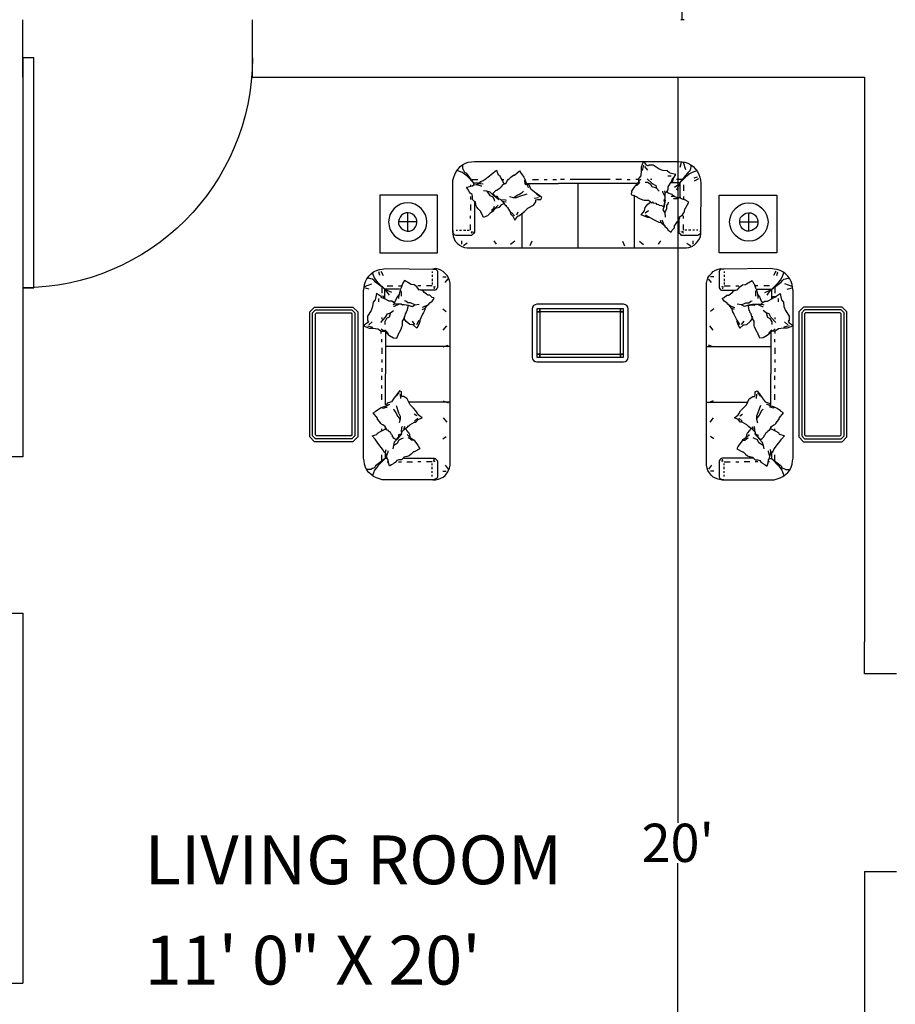
# Model space of a CAD drawing. Units: inches. Extents: x -113 to 5399, y -1393 to 3302.
# Tile 25 of 40: x 3844 to 3982, y 34 to 189. Entities that reach past the tile are written whole.
import ezdxf

# ---------------------------------------------------------------- set-up
doc = ezdxf.new("R2010")
doc.units = ezdxf.units.IN
doc.header["$MEASUREMENT"] = 0
doc.layers.add('24', color=7, linetype='Continuous')
for name, color, linetype, lineweight in [('A-ANNO-DIMS', 254, 'Continuous', 18), ('A-AREA-IDEN', 4, 'Continuous', 18), ('doors', 2, 'Continuous', 25), ('furniture', 131, 'Continuous', 18), ('walls', 1, 'Continuous', 25)]:
    doc.layers.add(name, color=color, linetype=linetype, lineweight=lineweight)
doc.styles.get("Standard").update_dxf_attribs({"font": 'arial.ttf'})
doc.dimstyles.get("Standard").update_dxf_attribs({"dimtxt": 6, "dimasz": 0.18, "dimexe": 0.18, "dimexo": 0.0625, "dimgap": 0.09, "dimtad": 0, "dimtih": 1, "dimtoh": 1, "dimdec": 1, "dimzin": 0, "dimdsep": 46, "dimlunit": 4, "dimtxsty": 'Standard', "dimblk": 'ARCHTICK', "dimcen": 0.09, "dimadec": 0, "dimazin": 0, "dimtfac": 1, "dimtdec": 1, "dimtofl": 0, "dimtmove": 0, "dimatfit": 3, "dimfxl": 1, "dimtolj": 1, "dimtzin": 0, "dimarcsym": 0})

# ---------------------------------------------------------------- blocks, each defined once
blk = doc.blocks.new('*U3')
for p, q in [((0, 0), (0, -6)), ((36, 0), (36, -6))]:
    blk.add_line(p, q)
blk.add_lwpolyline([(0, 0), (0, 36), (1.75, 36), (1.75, 0)], close=True)
blk.add_arc((0, 0), 36, 0, 90)
blk = doc.blocks.new('DL13712')
at = {"layer": '24'}
for p, q in [((33, 28.5), (-34, 28.5)), ((33.5, -29.5), (-10, -29.5))]:
    blk.add_line(p, q, dxfattribs=at)
blk = doc.blocks.new('DL13976')
at = {"layer": '24'}
for p, q in [((-18, 7.5), (-16, 11)), ((-16, 11), (-13.5, 14)), ((-13.5, 14), (-10.5, 16.5)), ((-10.5, 16.5), (-7, 18.5)), ((-7, 18.5), (-3.5, 19.5)), ((-3.5, 19.5), (0.5, 20)), ((0.5, 20), (4.5, 19.5)), ((4.5, 19.5), (8, 18.5)), ((8, 18.5), (11.5, 16.5)), ((11.5, 16.5), (14.5, 14)), ((14.5, 14), (17, 11)), ((17, 11), (19, 7.5)), ((-19.5, 0), (-19, 4)), ((-19, -4), (-19.5, 0)), ((-19, 4), (-18, 7.5)), ((-9, 2), (-8, 4.5)), ((-9, -0.5), (-9, 2)), ((-9, 0), (10, 0)), ((-8, 4.5), (-6.5, 6.5)), ((-6.5, 6.5), (-4.5, 8)), ((-5.5, 0), (6.5, 0)), ((-4.5, 8), (-2.5, 9)), ((-2.5, 9), (0, 9.5)), ((0, 9.5), (2.5, 9.5)), ((0.5, -9.5), (0.5, 9.5)), ((0.5, -6), (0.5, 6)), ((2.5, 9.5), (5, 8.5)), ((5, 8.5), (7, 7)), ((7, 7), (8.5, 5)), ((8.5, 5), (9.5, 3)), ((9.5, 3), (10, 0.5)), ((10, 0.5), (10, -2)), ((19, 7.5), (20, 4)), ((20, 4), (20.5, 0)), ((20.5, 0), (20, -4)), ((-18, -7.5), (-19, -4)), ((-16, -11), (-18, -7.5)), ((-8.5, -3), (-9, -0.5)), ((-7.5, -5), (-8.5, -3)), ((-6, -7), (-7.5, -5)), ((-4, -8.5), (-6, -7)), ((-1.5, -9.5), (-4, -8.5)), ((1, -9.5), (-1.5, -9.5)), ((3.5, -9), (1, -9.5)), ((5.5, -8), (3.5, -9)), ((7.5, -6.5), (5.5, -8)), ((9, -4.5), (7.5, -6.5)), ((10, -2), (9, -4.5)), ((19, -7.5), (17, -11)), ((20, -4), (19, -7.5)), ((-13.5, -14), (-16, -11)), ((-10.5, -16.5), (-13.5, -14)), ((-7, -18.5), (-10.5, -16.5)), ((-3.5, -19.5), (-7, -18.5)), ((0.5, -20), (-3.5, -19.5)), ((4.5, -19.5), (0.5, -20)), ((8, -18.5), (4.5, -19.5)), ((11.5, -16.5), (8, -18.5)), ((14.5, -14), (11.5, -16.5)), ((17, -11), (14.5, -14))]:
    blk.add_line(p, q, dxfattribs=at)
blk = doc.blocks.new('DL13329')
at = {"layer": '24'}
for p, q in [((0, 0), (0, -60)), ((60, 0), (0, 0)), ((60, -60), (60, 0)), ((0, -60), (60, -60))]:
    blk.add_line(p, q, dxfattribs=at)
blk = doc.blocks.new('DL13303')
at = {"layer": '24'}
for p, q in [((-70, 20), (-65, 25)), ((-67, 19), (-64, 22)), ((-65, 25), (65, 25)), ((-64, 22), (64, 22)), ((64, 22), (67, 19)), ((65, 25), (70, 20)), ((-70, -20), (-70, 20)), ((-67, -19), (-67, 19)), ((-64, 18), (-63, 19)), ((-64, -18), (-64, 18)), ((-63, 19), (63, 19)), ((63, 19), (64, 18)), ((64, 18), (64, -18)), ((67, 19), (67, -19)), ((70, 20), (70, -20)), ((-65, -25), (-70, -20)), ((-64, -22), (-67, -19)), ((-63, -19), (-64, -18)), ((63, -19), (-63, -19)), ((64, -18), (63, -19)), ((67, -19), (64, -22)), ((70, -20), (65, -25)), ((65, -25), (-65, -25)), ((64, -22), (-64, -22))]:
    blk.add_line(p, q, dxfattribs=at)
blk = doc.blocks.new('DL12701')
at = {"layer": '24'}
for p, q in [((-102, 40), (-99.5, 42)), ((-99.5, 42), (-96.5, 43.5)), ((-99, 40), (-99, 42)), ((-96.5, 43.5), (-93.5, 44.5)), ((-93.5, 44.5), (-90, 45)), ((-90, 45), (-87, 45.5)), ((-87, 45.5), (0, 45.5)), ((0, 45.5), (87, 45.5)), ((50, 45), (48, 39.5)), ((50.5, 41.5), (49, 36)), ((51.5, 44.5), (50, 45)), ((53.5, 41.5), (51.5, 44.5)), ((55.5, 40.5), (53.5, 41.5)), ((56, 41.5), (55.5, 40.5)), ((60.5, 41.5), (56, 41.5)), ((66.5, 37.5), (60.5, 41.5)), ((87, 45.5), (90.5, 45)), ((88.5, 39.5), (90, 44.5)), ((90.5, 45), (93.5, 44.5)), ((91.5, 44.5), (94, 37)), ((93.5, 44.5), (96.5, 43.5)), ((96.5, 43.5), (99.5, 42)), ((99.5, 42), (102, 40)), ((100, 40), (99.5, 42)), ((-108.5, 29), (-107.5, 32)), ((-107.5, 32), (-106, 35)), ((-106, 35), (-104, 37.5)), ((-102.5, 35), (-105, 36)), ((-104, 37.5), (-102, 40)), ((-99.5, 34), (-102.5, 35)), ((-97, 32), (-99.5, 34)), ((-99, 38), (-99, 40)), ((-98, 36), (-99, 38)), ((-97, 34), (-98, 36)), ((-95, 33), (-97, 34)), ((-95, 30.5), (-97, 32)), ((-87.5, 23), (-95, 33)), ((-71.5, 30.5), (-69.5, 32)), ((-69.5, 32), (-67.5, 33.5)), ((-67.5, 33.5), (-64, 36.5)), ((-64, 36.5), (-62.5, 31.5)), ((-62.5, 31.5), (-61, 31)), ((-61, 31), (-59.5, 28)), ((-49, 29), (-46.5, 31)), ((-46.5, 31), (-45.5, 31)), ((-45.5, 31), (-40, 35.5)), ((-40, 35.5), (-38.5, 33)), ((-38.5, 33), (-38, 32.5)), ((-38, 32.5), (-35.5, 29)), ((48, 35.5), (47.5, 30.5)), ((48, 39.5), (48, 35.5)), ((51.5, 40), (54.5, 36.5)), ((70.5, 36), (66.5, 37.5)), ((75, 35.5), (70.5, 36)), ((77.5, 33.5), (75, 35.5)), ((79, 33), (77.5, 33.5)), ((84, 32), (79, 33)), ((81.5, 28), (84, 32)), ((88.5, 23.5), (96, 33)), ((95.5, 30.5), (98, 32.5)), ((96, 33), (97.5, 34.5)), ((97.5, 34.5), (99, 36)), ((98, 32.5), (100.5, 34)), ((99, 36), (99.5, 38)), ((99.5, 38), (100, 40)), ((100.5, 34), (103, 35)), ((102, 40), (104.5, 37.5)), ((103, 35), (106, 36)), ((104.5, 37.5), (106.5, 35)), ((106.5, 35), (108, 32)), ((108, 32), (109, 29)), ((-109.5, 26), (-108.5, 29)), ((-109.5, 22.5), (-109.5, 26)), ((-109.5, -26.5), (-109.5, 22.5)), ((-87.5, 23), (-95, 30.5)), ((-91, 21), (-91, 19.5)), ((-89.5, 26.5), (-83.5, 26.5)), ((-89, 20), (-87.5, 21)), ((-87.5, 21), (-87.5, 23)), ((-81.5, 23), (-87.5, 23)), ((-87.5, 21), (-85, 21.5)), ((-85, 21.5), (-82, 22.5)), ((-85, 21.5), (-80.5, 20)), ((-82, 22.5), (-80.5, 24.5)), ((-82, 22.5), (-80.5, 22.5)), ((-80.5, 24.5), (-78, 25.5)), ((-80.5, 24.5), (-80.5, 23.5)), ((-80.5, 22.5), (-78, 22)), ((-78, 25.5), (-76, 27)), ((-77, 25.5), (-77, 25.5)), ((-76, 27), (-71.5, 30.5)), ((-59.5, 28), (-57.5, 24.5)), ((-58.5, 19.5), (-58, 21)), ((-58, 26.5), (-56.5, 26.5)), ((-58, 21), (-54.5, 23)), ((-57.5, 24.5), (-56.5, 22)), ((-56.5, 22.5), (-54.5, 22.5)), ((-54.5, 22.5), (-52.5, 25.5)), ((-54.5, 23), (-54.5, 22.5)), ((-54, 22.5), (-54, 22.5)), ((-52.5, 25.5), (-52, 26.5)), ((-52, 26.5), (-51, 27.5)), ((-51, 27.5), (-49, 29)), ((-35.5, 29), (-34.5, 27)), ((-34.5, 27), (-35, 24.5)), ((-35, 24.5), (-34.5, 23)), ((-34.5, 27), (-33.5, 24)), ((-34.5, 23), (-34, 21)), ((-33.5, 24), (-33, 22)), ((-30, 21), (-33, 22)), ((-33, 22), (-31.5, 19.5)), ((-32, 22.5), (0.5, 22.5)), ((-29.5, 19.5), (-30, 21)), ((-26.5, 26.5), (-20.5, 26.5)), ((-14.5, 26.5), (-11.5, 26.5)), ((-5.5, 26.5), (-1.5, 26.5)), ((44, 22.5), (0.5, 22.5)), ((6.5, 26.5), (2.5, 26.5)), ((15.5, 26.5), (12.5, 26.5)), ((27.5, 26.5), (21.5, 26.5)), ((33.5, 26.5), (36.5, 26.5)), ((43.5, 22), (41.5, 20)), ((43.5, 20.5), (41.5, 20)), ((42.5, 27), (45, 27)), ((45, 23.5), (43.5, 22)), ((45, 22), (43.5, 20.5)), ((45.5, 28), (45, 27)), ((45, 27), (45, 23.5)), ((45, 23.5), (46.5, 26)), ((46.5, 23.5), (45, 22)), ((47.5, 30.5), (45.5, 28)), ((46.5, 26), (47.5, 27)), ((54.5, 23.5), (52, 23.5)), ((54, 27.5), (59.5, 22.5)), ((58, 21.5), (54.5, 23.5)), ((59, 26.5), (57.5, 26.5)), ((59.5, 19), (58, 21.5)), ((59.5, 22.5), (63, 20.5)), ((63, 20.5), (64, 17.5)), ((79, 30), (75.5, 30)), ((76, 19), (79, 24)), ((80.5, 28), (79, 24)), ((79, 24), (81, 24.5)), ((79, 23.5), (88.5, 23.5)), ((81, 24.5), (81.5, 28)), ((82.5, 18.5), (88, 22.5)), ((90.5, 26.5), (84.5, 26.5)), ((85, 16), (88, 22.5)), ((88.5, 23.5), (95.5, 30.5)), ((88.5, 8), (88.5, 23.5)), ((92, 21), (92, 15)), ((103, 28.5), (106.5, 29.5)), ((107.5, 27.5), (103, 25)), ((109, 29), (109.5, 26)), ((109.5, 26), (110, 22.5)), ((110, 22.5), (109.5, -26.5)), ((-95, 18.5), (-92, 19.5)), ((-95, 18), (-95, 18.5)), ((-94, 16.5), (-95, 18)), ((-92.5, 14), (-94, 16.5)), ((-92, 13.5), (-92.5, 14)), ((-92, 19.5), (-89, 20)), ((-91.5, 12.5), (-92, 13.5)), ((-89.5, 11), (-91.5, 12.5)), ((-89, 9), (-89.5, 11)), ((-80.5, 20), (-79.5, 20)), ((-74, 14.5), (-77.5, 15)), ((-70.5, 13.5), (-74, 14.5)), ((-74, 14.5), (-71, 10)), ((-67.5, 10.5), (-70.5, 13.5)), ((-68, 12), (-67.5, 12.5)), ((-65, 9), (-68, 12)), ((-67.5, 12.5), (-66.5, 13.5)), ((-61.5, 5.5), (-67.5, 10.5)), ((-66.5, 13.5), (-64.5, 15.5)), ((-64.5, 15.5), (-63.5, 15.5)), ((-63.5, 15.5), (-62.5, 16.5)), ((-62.5, 16.5), (-60.5, 17.5)), ((-60.5, 17.5), (-59, 19.5)), ((-59, 19.5), (-58.5, 19.5)), ((-46.5, 7.5), (-42.5, 10.5)), ((-42.5, 10.5), (-40, 11.5)), ((-40, 11.5), (-37, 13.5)), ((-32.5, 11.5), (-40, 9)), ((-37, 13.5), (-36, 14.5)), ((-31.5, 19.5), (-31, 18)), ((-28.5, 16.5), (-29.5, 19.5)), ((-24.5, 13.5), (-28.5, 16.5)), ((-21, 11), (-24.5, 13.5)), ((-19, 8.5), (-22.5, 11.5)), ((-17, 8), (-21, 11)), ((38, 14), (37.5, 11)), ((37.5, 11), (43.5, 8.5)), ((40.5, 18.5), (38, 14.5)), ((38, 14.5), (38, 14)), ((41.5, 20), (40.5, 18.5)), ((64, 17.5), (59.5, 19)), ((64, 17.5), (66.5, 14.5)), ((70.5, 13.5), (70.5, 14.5)), ((73, 8.5), (70.5, 13.5)), ((73, 13), (72.5, 15)), ((73, 12.5), (75, 14.5)), ((73, 12.5), (73, 13)), ((73, 8.5), (73, 12.5)), ((76, 12.5), (74, 14)), ((75, 14.5), (76, 16)), ((75.5, 16), (76, 16.5)), ((76, 16), (76, 19)), ((80, 11), (76, 12.5)), ((80.5, 10.5), (80, 11)), ((83, 8.5), (80.5, 10.5)), ((-91, 9), (-91, 6)), ((-91, 0.5), (-91, -5.5)), ((-89, 8.5), (-89, 9)), ((-89, 6), (-89, 8.5)), ((-86.5, 3.5), (-89, 6)), ((-87, 3.5), (-87, -26.5)), ((-86, 3.5), (-86.5, 3.5)), ((-85.5, 0.5), (-86, 3.5)), ((-85.5, 0), (-85.5, 0.5)), ((-84.5, -2), (-85.5, 0)), ((-71, 10), (-68, 8.5)), ((-68, 8.5), (-66.5, 5.5)), ((-66.5, 5.5), (-66, 4)), ((-63, 9), (-65, 9)), ((-62.5, 0), (-63.5, -1)), ((-62, 6.5), (-63, 9)), ((-60, 6), (-62, 6.5)), ((-61, -2), (-58.5, 0.5)), ((-57.5, 3.5), (-60, 6)), ((-60, 6), (-55, 5.5)), ((-58.5, 0.5), (-55.5, 2)), ((-56.5, 3.5), (-57.5, 3.5)), ((-57.5, 3.5), (-56, 1.5)), ((-54, 3), (-56.5, 3.5)), ((-56, 1.5), (-55, 0)), ((-55, 5.5), (-54, 5)), ((-55, 0), (-52.5, -2.5)), ((-46.5, 7.5), (-50.5, 8.5)), ((-43.5, 7.5), (-46.5, 7.5)), ((-40, 9), (-43.5, 7.5)), ((-31.5, -3), (-25.5, 0)), ((-25.5, 0), (-23, 3.5)), ((-20.5, 7.5), (-25, 7)), ((-23, 5.5), (-21.5, 6)), ((-23, 3.5), (-23, 5.5)), ((-21.5, 6), (-18, 6)), ((-18, 6), (-17, 8)), ((43.5, 8.5), (44, 8)), ((44, 8), (47, 6.5)), ((47, 6.5), (49.5, 5.5)), ((49.5, 5.5), (51, 5)), ((51, 5), (52.5, 5)), ((52, -2.5), (55, 1)), ((52.5, 5), (55.5, 5)), ((55, 1), (57.5, 3)), ((55.5, 5), (55.5, 5)), ((55.5, 5), (59, 2.5)), ((59, 2.5), (60, 3.5)), ((60, 3.5), (60, 2.5)), ((60, 2.5), (63, 2)), ((63, 2), (64, 1)), ((64, 1), (66, 0.5)), ((66, 0.5), (66.5, 0)), ((66.5, 0), (69, -0.5)), ((71.5, -1), (72.5, 2.5)), ((72, 5), (73, 6.5)), ((73, 5.5), (72, -1)), ((72.5, 2.5), (72, 5)), ((73, 6.5), (73, 8.5)), ((74.5, -0.5), (76, 1.5)), ((76, 1.5), (76.5, 3)), ((80.5, 9), (79, 9)), ((83, 8.5), (80.5, 9)), ((84, 6.5), (81.5, 6.5)), ((85, 8), (83, 8.5)), ((85.5, 6.5), (84, 6.5)), ((88, 7.5), (85, 8)), ((88, 7.5), (85.5, 6.5)), ((90, 6.5), (88, 7.5)), ((94, 5), (90, 6.5)), ((92, 9), (92, 6)), ((95, 4.5), (94, 5)), ((94, -3), (97.5, 3)), ((97.5, 3), (95, 4.5)), ((-83, -4), (-84.5, -2)), ((-80.5, -6.5), (-83, -4)), ((-80.5, -7), (-80.5, -6.5)), ((-77.5, -13), (-80.5, -7)), ((-70.5, -8.5), (-73.5, -11)), ((-68.5, -7), (-70.5, -8.5)), ((-68.5, -4.5), (-67, -3)), ((-66.5, -4.5), (-68.5, -7)), ((-68.5, -7), (-68.5, -4.5)), ((-67, -3), (-66, -1)), ((-65.5, -3), (-66.5, -4.5)), ((-63.5, -1), (-65.5, -3)), ((-65.5, -3), (-62.5, -2.5)), ((-62.5, -2.5), (-61, -2)), ((-54, -0.5), (-53.5, -0.5)), ((-52.5, -2.5), (-49.5, -7.5)), ((-49.5, -7.5), (-49.5, -9)), ((-49.5, -9), (-47, -11.5)), ((-45.5, -11), (-48.5, -7.5)), ((-43, -10), (-41.5, -7)), ((-41, -11), (-38, -9)), ((-38, -9), (-35, -6.5)), ((-35, -6.5), (-31.5, -3)), ((48, -10), (51.5, -6)), ((52, -12), (48, -10)), ((51.5, -5.5), (52, -2.5)), ((51.5, -6), (51.5, -5.5)), ((52, -8), (55.5, -5.5)), ((52, -10), (56.5, -12.5)), ((69, -0.5), (70.5, -1)), ((70.5, -1), (71.5, -1)), ((72, -1), (70.5, -5)), ((70.5, -5), (72.5, -8)), ((72.5, -8), (74.5, -3.5)), ((72.5, -8), (73, -12.5)), ((74.5, -3.5), (74.5, -0.5)), ((89.5, -11), (91, -10)), ((91, -10), (92, -8.5)), ((92, -8.5), (93, -7)), ((93, -7), (93.5, -4)), ((93.5, -4), (94, -3)), ((-91, -14), (-91, -11)), ((-91, -26), (-91, -20)), ((-74.5, -11.5), (-77.5, -13)), ((-73.5, -11), (-74.5, -11.5)), ((-47, -11.5), (-45, -15.5)), ((-45, -15.5), (-42, -11.5)), ((-42, -11.5), (-41, -11)), ((55, -13), (52, -12)), ((56.5, -13), (55, -13)), ((62.5, -16), (56.5, -13)), ((64.5, -17), (62.5, -16)), ((64, -16.5), (64, -16.5)), ((66.5, -18), (64.5, -17)), ((69, -18.5), (66.5, -18)), ((67.5, -15.5), (68.5, -18)), ((68.5, -18), (69, -18.5)), ((69, -18.5), (72, -21)), ((70, -16.5), (69.5, -15.5)), ((72, -21), (70, -16.5)), ((82.5, -21.5), (83.5, -20)), ((83.5, -20), (85, -18)), ((85, -17.5), (87, -16.5)), ((85, -18), (85, -17.5)), ((87, -16.5), (88, -13)), ((87.5, -12.5), (89.5, -11)), ((88, -13), (87.5, -12.5)), ((87.5, -26.5), (87.5, -14.5)), ((92, -14), (92, -11)), ((92, -26), (92, -20)), ((-109.5, -28), (-109.5, -26.5)), ((-109.5, -26.5), (-109.5, -29.5)), ((-109, -29), (-109.5, -28)), ((-109.5, -29.5), (-109, -32.5)), ((-108.5, -30), (-109, -29)), ((-108, -31), (-108.5, -30)), ((-106, -26), (-104.5, -26)), ((-102.5, -26), (-100.5, -26)), ((-98.5, -26), (-96, -26)), ((-94.5, -26), (-92.5, -26)), ((-90.5, -27.5), (-88, -28)), ((-90.5, -28), (-90, -29)), ((-89, -30.5), (-90, -31.5)), ((-88, -30), (-89, -30.5)), ((-87.5, -29), (-88, -30)), ((-87, -28), (-87.5, -29)), ((-87, -26.5), (-87, -28)), ((72, -21), (73, -22.5)), ((73, -22.5), (74.5, -23.5)), ((74.5, -23.5), (76, -26)), ((76, -26), (79, -28)), ((79, -28), (79.5, -27.5)), ((79.5, -27.5), (80, -26)), ((80, -26), (82.5, -23.5)), ((82.5, -22.5), (82.5, -21.5)), ((82.5, -23.5), (82.5, -22.5)), ((87.5, -28), (87.5, -26.5)), ((87.5, -29), (87.5, -28)), ((88, -30), (87.5, -29)), ((89, -30.5), (88, -30)), ((91.5, -27.5), (89, -28)), ((90, -31.5), (89, -30.5)), ((91.5, -28), (91, -29)), ((95.5, -26), (93.5, -26)), ((99.5, -26), (97, -26)), ((103.5, -26), (101.5, -26)), ((107, -26), (105.5, -26)), ((109, -30), (108, -31)), ((109.5, -29), (109, -30)), ((110, -29.5), (109.5, -26.5)), ((109.5, -26.5), (109.5, -28)), ((109.5, -28), (109.5, -29)), ((109.5, -32.5), (110, -29.5)), ((-109, -32.5), (-108, -35)), ((-106.5, -31.5), (-108, -31)), ((-108, -35), (-107, -37.5)), ((-107, -37.5), (-105, -39.5)), ((-105.5, -31.5), (-106.5, -31.5)), ((-104.5, -31.5), (-105.5, -31.5)), ((-105, -39.5), (-102.5, -41.5)), ((-92, -31.5), (-104.5, -31.5)), ((-100.5, -37), (-100.5, -40.5)), ((-94.5, -39.5), (-98.5, -42.5)), ((-91, -31.5), (-92, -31.5)), ((-90, -31.5), (-91, -31.5)), ((-67, -37), (-64.5, -40.5)), ((-45, -37.5), (-49.5, -41)), ((-27.5, -37.5), (-29.5, -42.5)), ((28.5, -37.5), (30.5, -42.5)), ((46, -37.5), (50.5, -41)), ((68, -37), (65.5, -40.5)), ((91, -31.5), (90, -31.5)), ((92.5, -31.5), (91, -31.5)), ((104.5, -31.5), (92.5, -31.5)), ((95.5, -39.5), (99.5, -42.5)), ((101.5, -37), (101.5, -40.5)), ((103, -41.5), (105, -39.5)), ((106, -31.5), (104.5, -31.5)), ((105, -39.5), (107, -37.5)), ((107, -31.5), (106, -31.5)), ((108, -31), (107, -31.5)), ((107, -37.5), (108.5, -35)), ((108.5, -35), (109.5, -32.5)), ((-102.5, -41.5), (-100, -43)), ((-100, -43), (-97.5, -44)), ((-97.5, -44), (-94.5, -44.5)), ((-94.5, -44.5), (0, -44.5)), ((0, -44.5), (95, -44.5)), ((95, -44.5), (97.5, -44)), ((97.5, -44), (100.5, -43)), ((100.5, -43), (103, -41.5))]:
    blk.add_line(p, q, dxfattribs=at)
blk = doc.blocks.new('DL13707')
at = {"layer": '24'}
for p, q in [((0, -33.5), (0, 33.5)), ((-58.5, -33.5), (-58.5, 21.5)), ((58.5, -33.5), (58.5, 2))]:
    blk.add_line(p, q, dxfattribs=at)
blk = doc.blocks.new('DL13651')
at = {"layer": '24'}
for p, q in [((-50.5, 25), (-50, 27)), ((-50.5, -25), (-50.5, 25)), ((-50, 27), (-49, 28.5)), ((-49, 28.5), (-47.5, 29.5)), ((-47.5, 29.5), (-45.5, 30)), ((-45.5, 30), (44.5, 30)), ((-45.5, 24.5), (-45.5, 25)), ((-45.5, 25), (-45, 25)), ((-45.5, -24.5), (-45.5, 24.5)), ((-45, 25), (44, 25)), ((-45, 22), (44, 22)), ((-42.5, 22), (-45, 22)), ((-42.5, -24.5), (-42.5, 24.5)), ((-42.5, 24.5), (-42.5, 22)), ((41.5, 22), (41.5, 24.5)), ((41.5, 24.5), (41.5, -24.5)), ((44, 22), (41.5, 22)), ((44, 25), (44.5, 25)), ((44.5, 30), (46.5, 29.5)), ((44.5, 25), (44.5, 24.5)), ((44.5, 24.5), (44.5, -24.5)), ((46.5, 29.5), (48, 28.5)), ((48, 28.5), (49, 27)), ((49, 27), (49.5, 25)), ((49.5, 25), (49.5, -25)), ((-50, -27), (-50.5, -25)), ((-49, -28.5), (-50, -27)), ((-47.5, -29.5), (-49, -28.5)), ((-45.5, -30), (-47.5, -29.5)), ((-45.5, -25), (-45.5, -24.5)), ((-45, -25), (-45.5, -25)), ((44.5, -30), (-45.5, -30)), ((44, -22), (-45, -22)), ((-45, -22), (-42.5, -22)), ((44, -25), (-45, -25)), ((-42.5, -22), (-42.5, -24.5)), ((41.5, -24.5), (41.5, -22)), ((41.5, -22), (44, -22)), ((44.5, -25), (44, -25)), ((44.5, -24.5), (44.5, -25)), ((46.5, -29.5), (44.5, -30)), ((48, -28.5), (46.5, -29.5)), ((49, -27), (48, -28.5)), ((49.5, -25), (49, -27))]:
    blk.add_line(p, q, dxfattribs=at)
blk = doc.blocks.new('DL12263')
at = {"layer": '24'}
for p, q in [((-121, 40), (-118.5, 42)), ((-118.5, 42), (-115.5, 43.5)), ((-118, 40), (-118, 42)), ((-115.5, 43.5), (-112.5, 44.5)), ((-112.5, 44.5), (-109, 45)), ((-109, 45), (-106, 45.5)), ((-106, 45.5), (-19, 45.5)), ((-19, 45.5), (106.5, 45.5)), ((69.5, 45), (67.5, 39.5)), ((70, 41.5), (68.5, 36)), ((71, 44.5), (69.5, 45)), ((73, 41.5), (71, 44.5)), ((75, 40.5), (73, 41.5)), ((75.5, 41.5), (75, 40.5)), ((80, 41.5), (75.5, 41.5)), ((86, 37.5), (80, 41.5)), ((106.5, 45.5), (110, 45)), ((108, 39.5), (109.5, 44.5)), ((110, 45), (113, 44.5)), ((111, 44.5), (113.5, 37)), ((113, 44.5), (116, 43.5)), ((116, 43.5), (119, 42)), ((119, 42), (121.5, 40)), ((119.5, 40), (119, 42)), ((-127.5, 29), (-126.5, 32)), ((-126.5, 32), (-125, 35)), ((-125, 35), (-123, 37.5)), ((-121.5, 35), (-124, 36)), ((-123, 37.5), (-121, 40)), ((-118.5, 34), (-121.5, 35)), ((-116, 32), (-118.5, 34)), ((-118, 38), (-118, 40)), ((-117, 36), (-118, 38)), ((-116, 34), (-117, 36)), ((-114, 33), (-116, 34)), ((-114, 30.5), (-116, 32)), ((-106.5, 23), (-114, 33)), ((-90.5, 30.5), (-88.5, 32)), ((-88.5, 32), (-86.5, 33.5)), ((-86.5, 33.5), (-83, 36.5)), ((-83, 36.5), (-81.5, 31.5)), ((-81.5, 31.5), (-80, 31)), ((-80, 31), (-78.5, 28)), ((-68, 29), (-65.5, 31)), ((-65.5, 31), (-64.5, 31)), ((-64.5, 31), (-59, 35.5)), ((-59, 35.5), (-57.5, 33)), ((-57.5, 33), (-57, 32.5)), ((-57, 32.5), (-54.5, 29)), ((67.5, 35.5), (67, 30.5)), ((67.5, 39.5), (67.5, 35.5)), ((71, 40), (74, 36.5)), ((90, 36), (86, 37.5)), ((94.5, 35.5), (90, 36)), ((97, 33.5), (94.5, 35.5)), ((98.5, 33), (97, 33.5)), ((103.5, 32), (98.5, 33)), ((101, 28), (103.5, 32)), ((108, 23.5), (115.5, 33)), ((115, 30.5), (117.5, 32.5)), ((115.5, 33), (117, 34.5)), ((117, 34.5), (118.5, 36)), ((117.5, 32.5), (120, 34)), ((118.5, 36), (119, 38)), ((119, 38), (119.5, 40)), ((120, 34), (122.5, 35)), ((121.5, 40), (124, 37.5)), ((122.5, 35), (125.5, 36)), ((124, 37.5), (126, 35)), ((126, 35), (127.5, 32)), ((127.5, 32), (128.5, 29)), ((-128.5, 26), (-127.5, 29)), ((-128.5, 22.5), (-128.5, 26)), ((-128.5, -26.5), (-128.5, 22.5)), ((-106.5, 23), (-114, 30.5)), ((-110, 21), (-110, 19.5)), ((-108.5, 26.5), (-102.5, 26.5)), ((-108, 20), (-106.5, 21)), ((-106.5, 21), (-106.5, 23)), ((-100.5, 23), (-106.5, 23)), ((-106.5, 21), (-104, 21.5)), ((-104, 21.5), (-101, 22.5)), ((-104, 21.5), (-99.5, 20)), ((-101, 22.5), (-99.5, 24.5)), ((-101, 22.5), (-99.5, 22.5)), ((-99.5, 24.5), (-97, 25.5)), ((-99.5, 24.5), (-99.5, 23.5)), ((-99.5, 22.5), (-97, 22)), ((-97, 25.5), (-95, 27)), ((-96, 25.5), (-96, 25.5)), ((-95, 27), (-90.5, 30.5)), ((-78.5, 28), (-76.5, 24.5)), ((-77.5, 19.5), (-77, 21)), ((-77, 26.5), (-75.5, 26.5)), ((-77, 21), (-73.5, 23)), ((-76.5, 24.5), (-75.5, 22)), ((-75.5, 22.5), (-73.5, 22.5)), ((-73.5, 22.5), (-71.5, 25.5)), ((-73.5, 23), (-73.5, 22.5)), ((-73, 22.5), (-73, 22.5)), ((-71.5, 25.5), (-71, 26.5)), ((-71, 26.5), (-70, 27.5)), ((-70, 27.5), (-68, 29)), ((-54.5, 29), (-53.5, 27)), ((-53.5, 27), (-54, 24.5)), ((-54, 24.5), (-53.5, 23)), ((-53.5, 27), (-52.5, 24)), ((-53.5, 23), (-53, 21)), ((-52.5, 24), (-52, 22)), ((-49, 21), (-52, 22)), ((-52, 22), (-50.5, 19.5)), ((-51, 22.5), (-18.5, 22.5)), ((-48.5, 19.5), (-49, 21)), ((-45.5, 26.5), (-39.5, 26.5)), ((-33.5, 26.5), (-30.5, 26.5)), ((-24.5, 26.5), (-20.5, 26.5)), ((63.5, 22.5), (-18.5, 22.5)), ((-12.5, 26.5), (-16.5, 26.5)), ((35, 26.5), (-6.5, 26.5)), ((47, 26.5), (41, 26.5)), ((53, 26.5), (56, 26.5)), ((63, 22), (61, 20)), ((63, 20.5), (61, 20)), ((62, 27), (64.5, 27)), ((64.5, 23.5), (63, 22)), ((64.5, 22), (63, 20.5)), ((65, 28), (64.5, 27)), ((64.5, 27), (64.5, 23.5)), ((64.5, 23.5), (66, 26)), ((66, 23.5), (64.5, 22)), ((67, 30.5), (65, 28)), ((66, 26), (67, 27)), ((74, 23.5), (71.5, 23.5)), ((73.5, 27.5), (79, 22.5)), ((77.5, 21.5), (74, 23.5)), ((78.5, 26.5), (77, 26.5)), ((79, 19), (77.5, 21.5)), ((79, 22.5), (82.5, 20.5)), ((82.5, 20.5), (83.5, 17.5)), ((98.5, 30), (95, 30)), ((95.5, 19), (98.5, 24)), ((100, 28), (98.5, 24)), ((98.5, 24), (100.5, 24.5)), ((98.5, 23.5), (108, 23.5)), ((100.5, 24.5), (101, 28)), ((102, 18.5), (107.5, 22.5)), ((110, 26.5), (104, 26.5)), ((104.5, 16), (107.5, 22.5)), ((108, 23.5), (115, 30.5)), ((108, 8), (108, 23.5)), ((111.5, 21), (111.5, 15)), ((122.5, 28.5), (126, 29.5)), ((127, 27.5), (122.5, 25)), ((128.5, 29), (129, 26)), ((129, 26), (129.5, 22.5)), ((129.5, 22.5), (129, -26.5)), ((-114, 18.5), (-111, 19.5)), ((-114, 18), (-114, 18.5)), ((-113, 16.5), (-114, 18)), ((-111.5, 14), (-113, 16.5)), ((-111, 13.5), (-111.5, 14)), ((-111, 19.5), (-108, 20)), ((-110.5, 12.5), (-111, 13.5)), ((-108.5, 11), (-110.5, 12.5)), ((-108, 9), (-108.5, 11)), ((-99.5, 20), (-98.5, 20)), ((-93, 14.5), (-96.5, 15)), ((-89.5, 13.5), (-93, 14.5)), ((-93, 14.5), (-90, 10)), ((-86.5, 10.5), (-89.5, 13.5)), ((-87, 12), (-86.5, 12.5)), ((-84, 9), (-87, 12)), ((-86.5, 12.5), (-85.5, 13.5)), ((-80.5, 5.5), (-86.5, 10.5)), ((-85.5, 13.5), (-83.5, 15.5)), ((-83.5, 15.5), (-82.5, 15.5)), ((-82.5, 15.5), (-81.5, 16.5)), ((-81.5, 16.5), (-79.5, 17.5)), ((-79.5, 17.5), (-78, 19.5)), ((-78, 19.5), (-77.5, 19.5)), ((-65.5, 7.5), (-61.5, 10.5)), ((-61.5, 10.5), (-59, 11.5)), ((-59, 11.5), (-56, 13.5)), ((-51.5, 11.5), (-59, 9)), ((-56, 13.5), (-55, 14.5)), ((-50.5, 19.5), (-50, 18)), ((-47.5, 16.5), (-48.5, 19.5)), ((-43.5, 13.5), (-47.5, 16.5)), ((-40, 11), (-43.5, 13.5)), ((-38, 8.5), (-41.5, 11.5)), ((-36, 8), (-40, 11)), ((57.5, 14), (57, 11)), ((57, 11), (63, 8.5)), ((60, 18.5), (57.5, 14.5)), ((57.5, 14.5), (57.5, 14)), ((61, 20), (60, 18.5)), ((83.5, 17.5), (79, 19)), ((83.5, 17.5), (86, 14.5)), ((90, 13.5), (90, 14.5)), ((92.5, 8.5), (90, 13.5)), ((92.5, 13), (92, 15)), ((92.5, 12.5), (94.5, 14.5)), ((92.5, 12.5), (92.5, 13)), ((92.5, 8.5), (92.5, 12.5)), ((95.5, 12.5), (93.5, 14)), ((94.5, 14.5), (95.5, 16)), ((95, 16), (95.5, 16.5)), ((95.5, 16), (95.5, 19)), ((99.5, 11), (95.5, 12.5)), ((100, 10.5), (99.5, 11)), ((102.5, 8.5), (100, 10.5)), ((-110, 9), (-110, 6)), ((-110, 0.5), (-110, -5.5)), ((-108, 8.5), (-108, 9)), ((-108, 6), (-108, 8.5)), ((-105.5, 3.5), (-108, 6)), ((-106, 3.5), (-106, -26.5)), ((-105, 3.5), (-105.5, 3.5)), ((-104.5, 0.5), (-105, 3.5)), ((-104.5, 0), (-104.5, 0.5)), ((-103.5, -2), (-104.5, 0)), ((-90, 10), (-87, 8.5)), ((-87, 8.5), (-85.5, 5.5)), ((-85.5, 5.5), (-85, 4)), ((-82, 9), (-84, 9)), ((-81.5, 0), (-82.5, -1)), ((-81, 6.5), (-82, 9)), ((-79, 6), (-81, 6.5)), ((-80, -2), (-77.5, 0.5)), ((-76.5, 3.5), (-79, 6)), ((-79, 6), (-74, 5.5)), ((-77.5, 0.5), (-74.5, 2)), ((-75.5, 3.5), (-76.5, 3.5)), ((-76.5, 3.5), (-75, 1.5)), ((-73, 3), (-75.5, 3.5)), ((-75, 1.5), (-74, 0)), ((-74, 5.5), (-73, 5)), ((-74, 0), (-71.5, -2.5)), ((-65.5, 7.5), (-69.5, 8.5)), ((-62.5, 7.5), (-65.5, 7.5)), ((-59, 9), (-62.5, 7.5)), ((-50.5, -3), (-44.5, 0)), ((-44.5, 0), (-42, 3.5)), ((-39.5, 7.5), (-44, 7)), ((-42, 5.5), (-40.5, 6)), ((-42, 3.5), (-42, 5.5)), ((-40.5, 6), (-37, 6)), ((-37, 6), (-36, 8)), ((63, 8.5), (63.5, 8)), ((63.5, 8), (66.5, 6.5)), ((66.5, 6.5), (69, 5.5)), ((69, 5.5), (70.5, 5)), ((70.5, 5), (72, 5)), ((71.5, -2.5), (74.5, 1)), ((72, 5), (75, 5)), ((74.5, 1), (77, 3)), ((75, 5), (75, 5)), ((75, 5), (78.5, 2.5)), ((78.5, 2.5), (79.5, 3.5)), ((79.5, 3.5), (79.5, 2.5)), ((79.5, 2.5), (82.5, 2)), ((82.5, 2), (83.5, 1)), ((83.5, 1), (85.5, 0.5)), ((85.5, 0.5), (86, 0)), ((86, 0), (88.5, -0.5)), ((91, -1), (92, 2.5)), ((91.5, 5), (92.5, 6.5)), ((92.5, 5.5), (91.5, -1)), ((92, 2.5), (91.5, 5)), ((92.5, 6.5), (92.5, 8.5)), ((94, -0.5), (95.5, 1.5)), ((95.5, 1.5), (96, 3)), ((100, 9), (98.5, 9)), ((102.5, 8.5), (100, 9)), ((103.5, 6.5), (101, 6.5)), ((104.5, 8), (102.5, 8.5)), ((105, 6.5), (103.5, 6.5)), ((107.5, 7.5), (104.5, 8)), ((107.5, 7.5), (105, 6.5)), ((109.5, 6.5), (107.5, 7.5)), ((113.5, 5), (109.5, 6.5)), ((111.5, 9), (111.5, 6)), ((114.5, 4.5), (113.5, 5)), ((113.5, -3), (117, 3)), ((117, 3), (114.5, 4.5)), ((-102, -4), (-103.5, -2)), ((-99.5, -6.5), (-102, -4)), ((-99.5, -7), (-99.5, -6.5)), ((-96.5, -13), (-99.5, -7)), ((-89.5, -8.5), (-92.5, -11)), ((-87.5, -7), (-89.5, -8.5)), ((-87.5, -4.5), (-86, -3)), ((-85.5, -4.5), (-87.5, -7)), ((-87.5, -7), (-87.5, -4.5)), ((-86, -3), (-85, -1)), ((-84.5, -3), (-85.5, -4.5)), ((-82.5, -1), (-84.5, -3)), ((-84.5, -3), (-81.5, -2.5)), ((-81.5, -2.5), (-80, -2)), ((-73, -0.5), (-72.5, -0.5)), ((-71.5, -2.5), (-68.5, -7.5)), ((-68.5, -7.5), (-68.5, -9)), ((-68.5, -9), (-66, -11.5)), ((-64.5, -11), (-67.5, -7.5)), ((-62, -10), (-60.5, -7)), ((-60, -11), (-57, -9)), ((-57, -9), (-54, -6.5)), ((-54, -6.5), (-50.5, -3)), ((67.5, -10), (71, -6)), ((71.5, -12), (67.5, -10)), ((71, -5.5), (71.5, -2.5)), ((71, -6), (71, -5.5)), ((71.5, -8), (75, -5.5)), ((71.5, -10), (76, -12.5)), ((88.5, -0.5), (90, -1)), ((90, -1), (91, -1)), ((91.5, -1), (90, -5)), ((90, -5), (92, -8)), ((92, -8), (94, -3.5)), ((92, -8), (92.5, -12.5)), ((94, -3.5), (94, -0.5)), ((109, -11), (110.5, -10)), ((110.5, -10), (111.5, -8.5)), ((111.5, -8.5), (112.5, -7)), ((112.5, -7), (113, -4)), ((113, -4), (113.5, -3)), ((-110, -14), (-110, -11)), ((-110, -26), (-110, -20)), ((-93.5, -11.5), (-96.5, -13)), ((-92.5, -11), (-93.5, -11.5)), ((-66, -11.5), (-64, -15.5)), ((-64, -15.5), (-61, -11.5)), ((-61, -11.5), (-60, -11)), ((74.5, -13), (71.5, -12)), ((76, -13), (74.5, -13)), ((82, -16), (76, -13)), ((84, -17), (82, -16)), ((83.5, -16.5), (83.5, -16.5)), ((86, -18), (84, -17)), ((88.5, -18.5), (86, -18)), ((87, -15.5), (88, -18)), ((88, -18), (88.5, -18.5)), ((88.5, -18.5), (91.5, -21)), ((89.5, -16.5), (89, -15.5)), ((91.5, -21), (89.5, -16.5)), ((102, -21.5), (103, -20)), ((103, -20), (104.5, -18)), ((104.5, -17.5), (106.5, -16.5)), ((104.5, -18), (104.5, -17.5)), ((106.5, -16.5), (107.5, -13)), ((107, -12.5), (109, -11)), ((107.5, -13), (107, -12.5)), ((107, -26.5), (107, -14.5)), ((111.5, -14), (111.5, -11)), ((111.5, -26), (111.5, -20)), ((-128.5, -28), (-128.5, -26.5)), ((-128.5, -26.5), (-128.5, -29.5)), ((-128, -29), (-128.5, -28)), ((-128.5, -29.5), (-128, -32.5)), ((-127.5, -30), (-128, -29)), ((-127, -31), (-127.5, -30)), ((-125, -26), (-123.5, -26)), ((-121.5, -26), (-119.5, -26)), ((-117.5, -26), (-115, -26)), ((-113.5, -26), (-111.5, -26)), ((-109.5, -27.5), (-107, -28)), ((-109.5, -28), (-109, -29)), ((-108, -30.5), (-109, -31.5)), ((-107, -30), (-108, -30.5)), ((-106.5, -29), (-107, -30)), ((-106, -28), (-106.5, -29)), ((-106, -26.5), (-106, -28)), ((91.5, -21), (92.5, -22.5)), ((92.5, -22.5), (94, -23.5)), ((94, -23.5), (95.5, -26)), ((95.5, -26), (98.5, -28)), ((98.5, -28), (99, -27.5)), ((99, -27.5), (99.5, -26)), ((99.5, -26), (102, -23.5)), ((102, -22.5), (102, -21.5)), ((102, -23.5), (102, -22.5)), ((107, -28), (107, -26.5)), ((107, -29), (107, -28)), ((107.5, -30), (107, -29)), ((108.5, -30.5), (107.5, -30)), ((111, -27.5), (108.5, -28)), ((109.5, -31.5), (108.5, -30.5)), ((111, -28), (110.5, -29)), ((115, -26), (113, -26)), ((119, -26), (116.5, -26)), ((123, -26), (121, -26)), ((126.5, -26), (125, -26)), ((128.5, -30), (127.5, -31)), ((129, -29), (128.5, -30)), ((129.5, -29.5), (129, -26.5)), ((129, -26.5), (129, -28)), ((129, -28), (129, -29)), ((129, -32.5), (129.5, -29.5)), ((-128, -32.5), (-127, -35)), ((-125.5, -31.5), (-127, -31)), ((-127, -35), (-126, -37.5)), ((-126, -37.5), (-124, -39.5)), ((-124.5, -31.5), (-125.5, -31.5)), ((-123.5, -31.5), (-124.5, -31.5)), ((-124, -39.5), (-121.5, -41.5)), ((-111, -31.5), (-123.5, -31.5)), ((-119.5, -37), (-119.5, -40.5)), ((-113.5, -39.5), (-117.5, -42.5)), ((-110, -31.5), (-111, -31.5)), ((-109, -31.5), (-110, -31.5)), ((-86, -37), (-83.5, -40.5)), ((-64, -37.5), (-68.5, -41)), ((-46.5, -37.5), (-48.5, -42.5)), ((48, -37.5), (50, -42.5)), ((65.5, -37.5), (70, -41)), ((87.5, -37), (85, -40.5)), ((110.5, -31.5), (109.5, -31.5)), ((112, -31.5), (110.5, -31.5)), ((124, -31.5), (112, -31.5)), ((115, -39.5), (119, -42.5)), ((121, -37), (121, -40.5)), ((122.5, -41.5), (124.5, -39.5)), ((125.5, -31.5), (124, -31.5)), ((124.5, -39.5), (126.5, -37.5)), ((126.5, -31.5), (125.5, -31.5)), ((127.5, -31), (126.5, -31.5)), ((126.5, -37.5), (128, -35)), ((128, -35), (129, -32.5)), ((-121.5, -41.5), (-119, -43)), ((-119, -43), (-116.5, -44)), ((-116.5, -44), (-113.5, -44.5)), ((-113.5, -44.5), (-19, -44.5)), ((-19, -44.5), (114.5, -44.5)), ((114.5, -44.5), (117, -44)), ((117, -44), (120, -43)), ((120, -43), (122.5, -41.5))]:
    blk.add_line(p, q, dxfattribs=at)
blk = doc.blocks.new('U3M')
at = {"yscale": 10, "zscale": 10}
for name, p, xscale, rotation in [('DL13303', (1315, 2544), -10, 180), ('DL13976', (-270, 1769), 10, 90), ('DL13712', (1310, 1664), -10, 90), ('DL12263', (-445, 20), -10, 90), ('DL13707', (-335, 0), 10, 90), ('DL13651', (885, -25), 10, 270), ('DL13712', (1310, -1664), 10, 90), ('DL12701', (1315, -1779), 10, 180), ('DL13329', (50, -2064), 10, 180), ('DL13976', (-270, -1769), -10, 90)]:
    blk.add_blockref(name, p, dxfattribs=dict(at, xscale=xscale, rotation=rotation))
for name, p, xscale in [('DL12701', (1315, 1779), -10), ('DL13329', (50, 2064), -10), ('DL13303', (1315, -2544), 10)]:
    blk.add_blockref(name, p, dxfattribs=dict(at, xscale=xscale))
at = {"flags": 3}
for tag in ['AECLAY', 'AECGTYPE']:
    blk.add_attdef(tag, (0, 0), '', height=0.5, dxfattribs=at)
blk = doc.blocks.new('_ArchTick')
at = {"color": 0, "linetype": 'ByBlock', "const_width": 0.15}
blk.add_lwpolyline([(-0.5, -0.5), (0.5, 0.5)], dxfattribs=at)
blk = doc.blocks.new('*D95')
at = {"layer": 'A-ANNO-DIMS', "color": 0, "lineweight": -2, "transparency": 16777216}
for p, q in [((3948.45, 260.78), (3947.93, 260.78)), ((3948.11, 260.78), (3948.11, 227.93)), ((3948.11, 188.78), (3948.11, 221.62)), ((3948.45, 188.78), (3947.93, 188.78))]:
    blk.add_line(p, q, dxfattribs=at)
at = {"layer": 'Defpoints', "color": 0, "transparency": 16777216}
for p in [(3948.51, 260.78), (3948.11, 188.78), (3948.51, 188.78)]:
    blk.add_point(p, dxfattribs=at)
at = {"layer": 'A-ANNO-DIMS', "color": 0, "lineweight": -2, "transparency": 16777216, "xscale": 0.18, "yscale": 0.18, "zscale": 0.18}
for p, rotation in [((3948.11, 260.78), 90), ((3948.11, 188.78), 270)]:
    blk.add_blockref('_ArchTick', p, dxfattribs=dict(at, rotation=rotation))
at = {"layer": 'A-ANNO-DIMS', "color": 0, "transparency": 16777216, "insert": (3948.11, 224.78), "char_height": 6, "attachment_point": 5}
blk.add_mtext("\\A1;6'", dxfattribs=at)
blk = doc.blocks.new('*D101')
at = {"layer": 'A-ANNO-DIMS', "color": 0, "lineweight": -2, "transparency": 16777216}
for p, q in [((3947.43, 179.78), (3947.43, 62.93)), ((3947.5, 179.78), (3947.61, 179.78)), ((3947.43, -60.22), (3947.43, 56.62)), ((3947.5, -60.22), (3947.61, -60.22))]:
    blk.add_line(p, q, dxfattribs=at)
at = {"layer": 'Defpoints', "color": 0, "transparency": 16777216}
for p in [(3947.43, 179.78), (3947.43, 179.78), (3947.43, -60.22)]:
    blk.add_point(p, dxfattribs=at)
at = {"layer": 'A-ANNO-DIMS', "color": 0, "lineweight": -2, "transparency": 16777216, "xscale": 0.18, "yscale": 0.18, "zscale": 0.18}
for p, rotation in [((3947.43, 179.78), 90), ((3947.43, -60.22), 270)]:
    blk.add_blockref('_ArchTick', p, dxfattribs=dict(at, rotation=rotation))
at = {"layer": 'A-ANNO-DIMS', "color": 0, "transparency": 16777216, "insert": (3947.43, 59.78), "char_height": 6, "attachment_point": 5}
blk.add_mtext("\\A1;20'", dxfattribs=at)
blk = doc.blocks.new('*D210')
at = {"layer": 'A-ANNO-DIMS', "color": 0, "lineweight": -2, "transparency": 16777216}
for p, q in [((3839.79, 561.28), (4159.21, 561.28)), ((4159.03, 561.28), (4159.03, 230.43)), ((4159.03, -106.72), (4159.03, 224.12)), ((3839.79, -106.72), (4159.21, -106.72))]:
    blk.add_line(p, q, dxfattribs=at)
at = {"layer": 'Defpoints', "color": 0, "transparency": 16777216}
for p in [(3839.73, 561.28), (4159.03, 561.28), (3839.73, -106.72)]:
    blk.add_point(p, dxfattribs=at)
at = {"layer": 'A-ANNO-DIMS', "color": 0, "lineweight": -2, "transparency": 16777216, "xscale": 0.18, "yscale": 0.18, "zscale": 0.18}
for p, rotation in [((4159.03, 561.28), 90), ((4159.03, -106.72), 270)]:
    blk.add_blockref('_ArchTick', p, dxfattribs=dict(at, rotation=rotation))
at = {"layer": 'A-ANNO-DIMS', "color": 0, "transparency": 16777216, "insert": (4159.03, 227.28), "char_height": 6, "attachment_point": 5}
blk.add_mtext('\\A1;55\'-8"', dxfattribs=at)

msp = doc.modelspace()

# ---------------------------------------------------------------- linework, layer by layer
at = {"layer": 'walls'}
for p, q in [((3844.73, 179.78), (3844.73, 188.78)), ((3880.73, 179.78), (3880.73, 188.78)), ((3844.73, 179.78), (3844.73, 120.28)), ((3880.73, 179.78), (3976.73, 179.78)), ((3976.73, 179.78), (3976.73, 91.28)), ((3844.73, 120.28), (3820.73, 120.28)), ((3839.73, 95.78), (3844.73, 95.78)), ((3844.73, 95.78), (3844.73, 37.78)), ((3976.73, 86.28), (3976.73, 91.28)), ((3981.73, 86.28), (3976.73, 86.28)), ((3976.73, 55.28), (3976.73, -19.22)), ((3976.73, 55.28), (3981.73, 55.28)), ((3839.73, 37.78), (3844.73, 37.78))]:
    msp.add_line(p, q, dxfattribs=at)

# ---------------------------------------------------------------- block references
at = {"layer": 'doors', "xscale": -1, "rotation": 180}
msp.add_blockref('*U3', (3844.73, 182.78), dxfattribs=at)
at = {"layer": 'furniture', "xscale": -0.0150724250692195, "yscale": 0.0150724250692195, "zscale": 0.0150724250692195, "rotation": 90}
msp.add_blockref('U3M', (3931.83, 153.01), dxfattribs=at)

# ---------------------------------------------------------------- texts
at = {"layer": 'A-AREA-IDEN'}
for s, p in [('LIVING ROOM', (3863.85, 53.29)), ('11\' 0" X 20\'', (3863.85, 37.57))]:
    msp.add_text(s, height=7.6473, dxfattribs=at).set_placement(p)

# ---------------------------------------------------------------- dimensions: what is measured, and where the dimension line sits
at = {"layer": 'A-ANNO-DIMS'}
for base, p1, p2, override, picture, middle in [((4159.03, 561.28), (3839.73, -106.72), (3839.73, 561.28), {"dimdec": 1, "dimlfac": 1, "dimrnd": 0, "dimzin": 1, "dimdsep": 46, "dimlunit": 4, "dimfrac": 2}, '*D210', (4159.03, 227.28)), ((3948.11, 188.78), (3948.51, 260.78), (3948.51, 188.78), {"dimclrd": 0, "dimclre": 0, "dimclrt": 0}, '*D95', (3948.11, 224.78)), ((3947.43, 179.78), (3947.43, -60.22), (3947.43, 179.78), {"dimclrd": 0, "dimclre": 0, "dimclrt": 0}, '*D101', (3947.43, 59.78))]:
    dim = msp.add_linear_dim(base=base, p1=p1, p2=p2, angle=90, dimstyle='Standard', override=override, dxfattribs=at)
    dim.commit()
    dim.dimension.update_dxf_attribs({"geometry": picture, "text_midpoint": middle})

doc.saveas('drawing.dxf')
